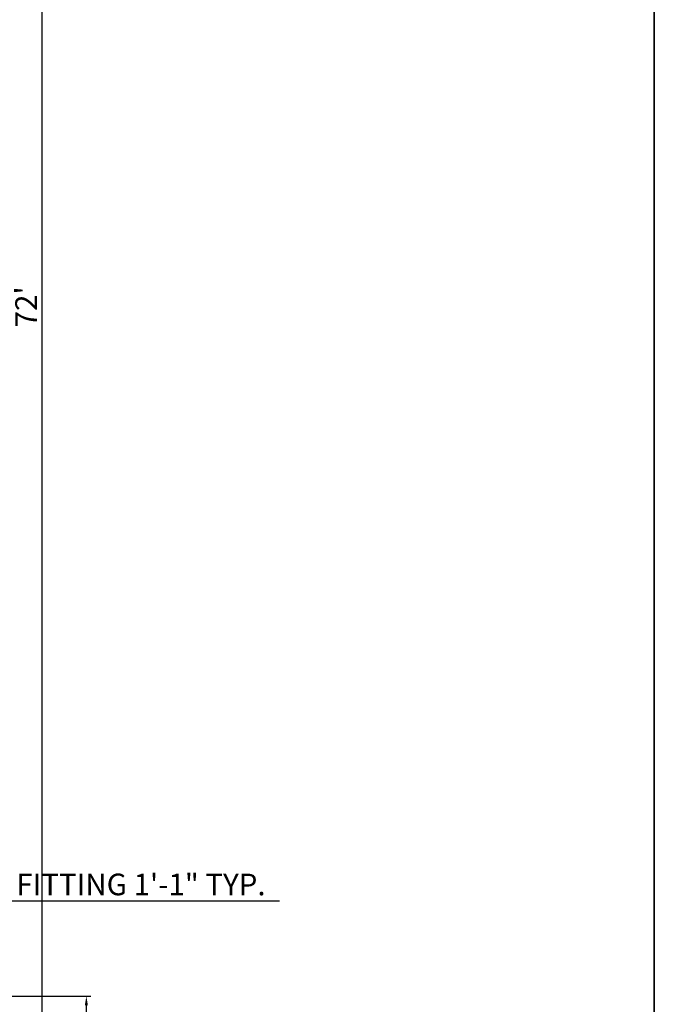
# Model space of a CAD drawing. Units: inches. Extents: x 2123 to 2977, y 1464 to 2698.
# Tile 6 of 10: x 2801 to 2977, y 1923 to 2196. Entities that reach past the tile are written whole.
import ezdxf

# ---------------------------------------------------------------- set-up
doc = ezdxf.new("R2010")
doc.units = ezdxf.units.IN
doc.layers.add('A-ANNO-DIMS', color=2, linetype='Continuous', lineweight=18)
doc.layers.add('A-ANNO-TTLB', color=7, linetype='Continuous', lineweight=35)
doc.styles.get("Standard").update_dxf_attribs({"font": 'arial.ttf'})
doc.dimstyles.new('ISO-25', dxfattribs={"dimtxt": 6, "dimasz": 2.5, "dimexe": 1.25, "dimexo": 0.625, "dimtad": 1, "dimdec": 0, "dimlunit": 3, "dimtxsty": 'Standard', "dimcen": 2.5, "dimadec": 0, "dimazin": 0, "dimtfac": 1, "dimtdec": 0, "dimtmove": 0, "dimatfit": 3, "dimfxl": 1, "dimarcsym": 0})

# ---------------------------------------------------------------- blocks, each defined once
blk = doc.blocks.new('*D9')
at = {"layer": 'A-ANNO-DIMS', "color": 0, "lineweight": -2, "transparency": 16777216}
for p, q in [((2767.56, 2548.37), (2808.58, 2548.37)), ((2807.33, 2545.87), (2807.33, 1686.46)), ((2767.56, 1683.96), (2808.58, 1683.96))]:
    blk.add_line(p, q, dxfattribs=at)
at = {"layer": 'A-ANNO-DIMS', "color": 0, "transparency": 16777216}
for points in [[(2806.91, 2545.87), (2807.74, 2545.87), (2807.33, 2548.37)], [(2806.91, 1686.46), (2807.74, 1686.46), (2807.33, 1683.96)]]:
    blk.add_solid(points, dxfattribs=at)
at = {"layer": 'Defpoints', "color": 0, "transparency": 16777216}
for p in [(2766.94, 2548.37), (2766.94, 1683.96), (2807.33, 1683.96)]:
    blk.add_point(p, dxfattribs=at)
at = {"layer": 'A-ANNO-DIMS', "color": 0, "transparency": 16777216, "insert": (2803.69, 2116.16), "char_height": 6, "attachment_point": 5, "rotation": 90}
blk.add_mtext("72'", dxfattribs=at)
blk = doc.blocks.new('*D44')
at = {"layer": 'A-ANNO-DIMS', "color": 0, "lineweight": -2, "transparency": 16777216}
for p, q in [((2744.82, 1952.72), (2744.82, 1950.13)), ((2747.32, 1951.38), (2755.44, 1951.38)), ((2757.94, 1952.72), (2757.94, 1950.13)), ((2757.94, 1951.38), (2873.2, 1951.38))]:
    blk.add_line(p, q, dxfattribs=at)
at = {"layer": 'A-ANNO-DIMS', "color": 0, "transparency": 16777216}
for points in [[(2747.32, 1951.79), (2747.32, 1950.96), (2744.82, 1951.38)], [(2755.44, 1951.79), (2755.44, 1950.96), (2757.94, 1951.38)]]:
    blk.add_solid(points, dxfattribs=at)
at = {"layer": 'Defpoints', "color": 0, "transparency": 16777216}
for p in [(2744.82, 1953.34), (2757.94, 1953.34), (2757.94, 1951.38)]:
    blk.add_point(p, dxfattribs=at)
at = {"layer": 'A-ANNO-DIMS', "color": 0, "transparency": 16777216, "insert": (2816.82, 1955.11), "char_height": 6, "attachment_point": 5}
blk.add_mtext('SHOWER FITTING 1\'-1" TYP.', dxfattribs=at)
blk = doc.blocks.new('*D55')
at = {"layer": 'A-ANNO-DIMS', "color": 0, "lineweight": -2, "transparency": 16777216}
for p, q in [((2758.56, 1924.87), (2820.89, 1924.87)), ((2819.64, 1695.76), (2819.64, 1922.37)), ((2758.56, 1693.26), (2820.89, 1693.26))]:
    blk.add_line(p, q, dxfattribs=at)
at = {"layer": 'A-ANNO-DIMS', "color": 0, "transparency": 16777216}
for points in [[(2819.22, 1922.37), (2820.05, 1922.37), (2819.64, 1924.87)], [(2819.22, 1695.76), (2820.05, 1695.76), (2819.64, 1693.26)]]:
    blk.add_solid(points, dxfattribs=at)
at = {"layer": 'Defpoints', "color": 0, "transparency": 16777216}
for p in [(2757.94, 1924.87), (2819.64, 1924.87), (2757.94, 1693.26)]:
    blk.add_point(p, dxfattribs=at)
at = {"layer": 'A-ANNO-DIMS', "color": 0, "transparency": 16777216, "insert": (2815.91, 1809.06), "char_height": 6, "attachment_point": 5, "rotation": 90}
blk.add_mtext('19\'-3 1/2"', dxfattribs=at)

msp = doc.modelspace()

# ---------------------------------------------------------------- linework, layer by layer
at = {"layer": 'A-ANNO-TTLB'}
msp.add_lwpolyline([(2123.3, 2697.62), (2977.18, 2697.62), (2977.18, 1463.53), (2123.3, 1463.53)], close=True, dxfattribs=at)

# ---------------------------------------------------------------- dimensions: what is measured, and where the dimension line sits
at = {"layer": 'A-ANNO-DIMS'}
for base, p1, p2, override, picture, middle in [((2807.33, 1683.96), (2766.94, 2548.37), (2766.94, 1683.96), {"dimclrd": 0, "dimclre": 0, "dimclrt": 0}, '*D9', (2803.69, 2116.16)), ((2819.64, 1924.87), (2757.94, 1693.26), (2757.94, 1924.87), {"dimdec": 1, "dimlfac": 1, "dimrnd": 0, "dimzin": 1, "dimdsep": 46, "dimlunit": 4, "dimfrac": 2}, '*D55', (2815.91, 1809.06))]:
    dim = msp.add_linear_dim(base=base, p1=p1, p2=p2, angle=90, dimstyle='ISO-25', override=override, dxfattribs=at)
    dim.commit()
    dim.dimension.update_dxf_attribs({"geometry": picture, "text_midpoint": middle})
dim = msp.add_linear_dim(base=(2757.94, 1951.38), p1=(2744.82, 1953.34), p2=(2757.94, 1953.34), text='SHOWER FITTING <> TYP.', dimstyle='ISO-25', override={"dimdec": 1, "dimlfac": 1, "dimrnd": 0, "dimzin": 1, "dimdsep": 46, "dimlunit": 4, "dimfrac": 2}, dxfattribs=at)
dim.commit()
dim.dimension.update_dxf_attribs({"geometry": '*D44', "text_midpoint": (2816.82, 1955.11)})

doc.saveas('drawing.dxf')
